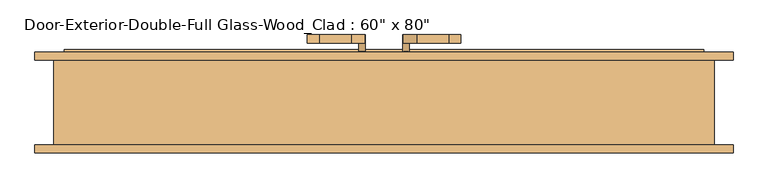
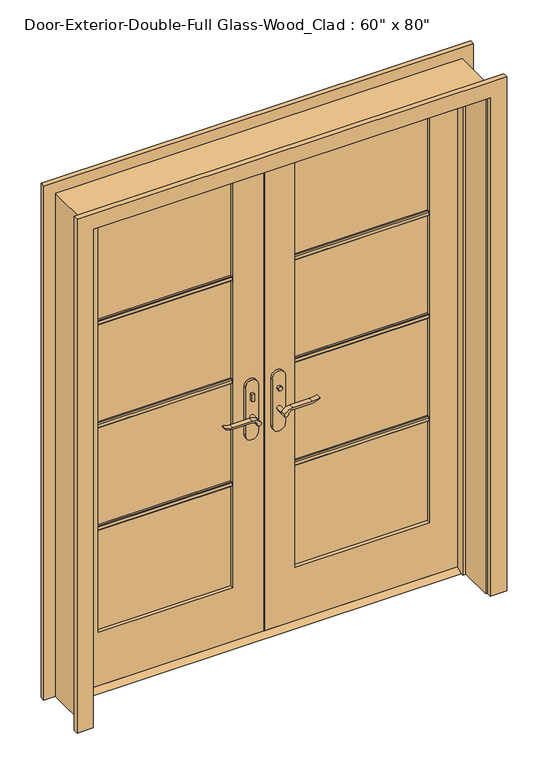
"""IFC4 building model written with IfcOpenShell, lengths in millimetres: door geometry."""

from ifc_helpers import new_model, si_unit, point, frame, frame_2d, origin, place, context, project, spatial, polyline, circle_curve, trimmed, segment, composite_curve, outline, extrude, faceted_brep, source, transform, mapped, element, save


def door_b03bd389(model_context):
    return source(origin(), model_context, "Body", "SolidModel", [
        extrude(outline(polyline([(63.5, 12.7), (98.425, 12.7), (123.825, 0.0), (38.1, 0.0), (63.5, 12.7)])), frame((-762.0, 0.0, 0.0), z_axis=(1.0, 0.0, 0.0), x_axis=(0.0, 1.0, 0.0)), (0.0, 0.0, 1.0), 1524.0),
        extrude(outline(polyline([(-47.4019111, 43.5), (-57.4019111, 43.5), (-57.4019111, 53.5), (-47.4019111, 53.5), (-47.4019111, 43.5)])), frame((0.0, 0.0, 981.9), z_axis=(0.0, 0.0, 1.0), x_axis=(1.0, 0.0, 0.0)), (0.0, 0.0, 1.0), 30.0),
        extrude(outline(composite_curve([segment(trimmed(circle_curve(frame_2d((996.9, -52.4019111)), 8.0), [point((996.9, -60.4019111))], [point((996.9, -44.4019111))], False, "CARTESIAN"), True, "CONTINUOUS"), segment(trimmed(circle_curve(frame_2d((996.9, -52.4019111)), 8.0), [point((996.9, -44.4019111))], [point((996.9, -60.4019111))], False, "CARTESIAN"), True, "CONTINUOUS")], self_intersect=False)), frame((0.0, 108.425, 0.0), z_axis=(0.0, 1.0, 0.0), x_axis=(0.0, 0.0, 1.0)), (0.0, 0.0, 1.0), 10.0),
        extrude(outline(composite_curve([segment(trimmed(circle_curve(frame_2d((897.1555521, -76.0694241)), 37.2832219), [point((919.0523287, -45.8937749))], [point((934.4, -77.7693445))], False, "CARTESIAN"), True, "CONTINUOUS"), segment(polyline([(934.4, -77.7693445), (934.4, -154.045502)]), True, "CONTINUOUS"), segment(trimmed(circle_curve(frame_2d((1017.6850638, -153.9791202)), 83.2850902), [point((934.4, -154.045502))], [point((939.4, -182.4019111))], True, "CARTESIAN"), True, "CONTINUOUS"), segment(polyline([(939.4, -182.4019111), (936.6135558, -182.4019111)]), True, "CONTINUOUS"), segment(trimmed(circle_curve(frame_2d((986.6709207, -150.4622499)), 59.3791355), [point((936.6135558, -182.4019111))], [point((927.4, -154.045502))], False, "CARTESIAN"), True, "CONTINUOUS"), segment(polyline([(927.4, -154.045502), (927.4, -77.7881013)]), True, "CONTINUOUS"), segment(trimmed(circle_curve(frame_2d((909.2738613, -77.7881013)), 18.1261387), [point((927.4, -77.7881013))], [point((914.4, -60.4019111))], True, "CARTESIAN"), True, "CONTINUOUS"), segment(trimmed(circle_curve(frame_2d((914.4, -52.4019111)), 8.0), [point((914.4, -60.4019111))], [point((919.0523287, -45.8937749))], False, "CARTESIAN"), True, "CONTINUOUS")], self_intersect=False)), frame((0.0, 3.5, 0.0), z_axis=(0.0, 1.0, 0.0), x_axis=(0.0, 0.0, 1.0)), (0.0, 0.0, 1.0), 20.0),
        extrude(outline(composite_curve([segment(trimmed(circle_curve(frame_2d((914.4, -52.4019111)), 8.0), [point((914.3999903, -60.4019111))], [point((919.0523287, -45.8937749))], False, "CARTESIAN"), True, "CONTINUOUS"), segment(trimmed(circle_curve(frame_2d((897.1555521, -76.0694241)), 37.2832219), [point((919.0523287, -45.8937749))], [point((934.4, -77.7693445))], False, "CARTESIAN"), True, "CONTINUOUS"), segment(polyline([(934.4, -77.7693445), (934.4, -154.045502)]), True, "CONTINUOUS"), segment(trimmed(circle_curve(frame_2d((1017.6850638, -153.9791202)), 83.2850902), [point((934.4, -154.045502))], [point((939.4, -182.4019111))], True, "CARTESIAN"), True, "CONTINUOUS"), segment(polyline([(939.4, -182.4019111), (936.6135558, -182.4019111)]), True, "CONTINUOUS"), segment(trimmed(circle_curve(frame_2d((986.6709207, -150.4622499)), 59.3791355), [point((936.6135558, -182.4019111))], [point((927.4, -154.045502))], False, "CARTESIAN"), True, "CONTINUOUS"), segment(polyline([(927.4, -154.045502), (927.4, -77.788099)]), True, "CONTINUOUS"), segment(trimmed(circle_curve(frame_2d((909.2738682, -77.788099)), 18.1261318), [point((927.4, -77.788099))], [point((914.3999903, -60.4019111))], True, "CARTESIAN"), True, "CONTINUOUS")], self_intersect=False)), frame((0.0, 138.425, 0.0), z_axis=(0.0, 1.0, 0.0), x_axis=(0.0, 0.0, 1.0)), (0.0, 0.0, 1.0), 20.0),
        extrude(outline(composite_curve([segment(trimmed(circle_curve(frame_2d((914.4, -52.4019111)), 8.0), [point((914.4, -60.4019111))], [point((914.4, -44.4019111))], False, "CARTESIAN"), True, "CONTINUOUS"), segment(trimmed(circle_curve(frame_2d((914.4, -52.4019111)), 8.0), [point((914.4, -44.4019111))], [point((914.4, -60.4019111))], False, "CARTESIAN"), True, "CONTINUOUS")], self_intersect=False)), frame((0.0, 23.5, 0.0), z_axis=(0.0, 1.0, 0.0), x_axis=(0.0, 0.0, 1.0)), (0.0, 0.0, 1.0), 30.0),
        extrude(outline(composite_curve([segment(trimmed(circle_curve(frame_2d((914.4, -52.4019111)), 8.0), [point((914.4, -60.4019111))], [point((914.4, -44.4019111))], False, "CARTESIAN"), True, "CONTINUOUS"), segment(trimmed(circle_curve(frame_2d((914.4, -52.4019111)), 8.0), [point((914.4, -44.4019111))], [point((914.4, -60.4019111))], False, "CARTESIAN"), True, "CONTINUOUS")], self_intersect=False)), frame((0.0, 108.425, 0.0), z_axis=(0.0, 1.0, 0.0), x_axis=(0.0, 0.0, 1.0)), (0.0, 0.0, 1.0), 30.0),
        extrude(outline(composite_curve([segment(polyline([(844.4, -27.4019111), (1039.4, -27.4019111)]), True, "CONTINUOUS"), segment(trimmed(circle_curve(frame_2d((1039.4, -52.4019111)), 25.0), [point((1039.4, -27.4019111))], [point((1039.4, -77.4019111))], False, "CARTESIAN"), True, "CONTINUOUS"), segment(polyline([(1039.4, -77.4019111), (844.4, -77.4019111)]), True, "CONTINUOUS"), segment(trimmed(circle_curve(frame_2d((844.4, -52.4019111)), 25.0), [point((844.4, -77.4019111))], [point((844.4, -27.4019111))], False, "CARTESIAN"), True, "CONTINUOUS")], self_intersect=False)), frame((0.0, 53.5, 0.0), z_axis=(0.0, 1.0, 0.0), x_axis=(0.0, 0.0, 1.0)), (0.0, 0.0, 1.0), 10.0),
        extrude(outline(composite_curve([segment(polyline([(844.4, -27.4019111), (1039.4, -27.4019111)]), True, "CONTINUOUS"), segment(trimmed(circle_curve(frame_2d((1039.4, -52.4019111)), 25.0), [point((1039.4, -27.4019111))], [point((1039.4, -77.4019111))], False, "CARTESIAN"), True, "CONTINUOUS"), segment(polyline([(1039.4, -77.4019111), (844.4, -77.4019111)]), True, "CONTINUOUS"), segment(trimmed(circle_curve(frame_2d((844.4, -52.4019111)), 25.0), [point((844.4, -77.4019111))], [point((844.4, -27.4019111))], False, "CARTESIAN"), True, "CONTINUOUS")], self_intersect=False)), frame((0.0, 98.425, 0.0), z_axis=(0.0, 1.0, 0.0), x_axis=(0.0, 0.0, 1.0)), (0.0, 0.0, 1.0), 10.0),
        extrude(outline(polyline([(47.3875, 118.425), (57.3875, 118.425), (57.3875, 108.425), (47.3875, 108.425), (47.3875, 118.425)])), frame((0.0, 0.0, 981.9), z_axis=(0.0, 0.0, 1.0), x_axis=(1.0, 0.0, 0.0)), (0.0, 0.0, 1.0), 30.0),
        extrude(outline(composite_curve([segment(trimmed(circle_curve(frame_2d((996.9, 52.3875)), 8.0), [point((996.9, 60.3875))], [point((996.9, 44.3875))], False, "CARTESIAN"), True, "CONTINUOUS"), segment(trimmed(circle_curve(frame_2d((996.9, 52.3875)), 8.0), [point((996.9, 44.3875))], [point((996.9, 60.3875))], False, "CARTESIAN"), True, "CONTINUOUS")], self_intersect=False)), frame((0.0, 43.5, 0.0), z_axis=(0.0, 1.0, 0.0), x_axis=(0.0, 0.0, 1.0)), (0.0, 0.0, 1.0), 10.0),
        extrude(outline(composite_curve([segment(trimmed(circle_curve(frame_2d((914.4, 52.3875)), 8.0), [point((919.0523287, 45.8793637))], [point((914.4, 60.3875))], False, "CARTESIAN"), True, "CONTINUOUS"), segment(trimmed(circle_curve(frame_2d((909.2738613, 77.7736901)), 18.1261387), [point((914.4, 60.3875))], [point((927.4, 77.7736901))], True, "CARTESIAN"), True, "CONTINUOUS"), segment(polyline([(927.4, 77.7736901), (927.4, 154.0310909)]), True, "CONTINUOUS"), segment(trimmed(circle_curve(frame_2d((986.6709207, 150.4478388)), 59.3791355), [point((927.4, 154.0310909))], [point((936.6135558, 182.3875))], False, "CARTESIAN"), True, "CONTINUOUS"), segment(polyline([(936.6135558, 182.3875), (939.4, 182.3875)]), True, "CONTINUOUS"), segment(trimmed(circle_curve(frame_2d((1017.6850638, 153.9647091)), 83.2850902), [point((939.4, 182.3875))], [point((934.4, 154.0310909))], True, "CARTESIAN"), True, "CONTINUOUS"), segment(polyline([(934.4, 154.0310909), (934.4, 77.7549333)]), True, "CONTINUOUS"), segment(trimmed(circle_curve(frame_2d((897.1555521, 76.0550129)), 37.2832219), [point((934.4, 77.7549333))], [point((919.0523287, 45.8793637))], False, "CARTESIAN"), True, "CONTINUOUS")], self_intersect=False)), frame((0.0, 138.425, 0.0), z_axis=(0.0, 1.0, 0.0), x_axis=(0.0, 0.0, 1.0)), (0.0, 0.0, 1.0), 20.0),
        extrude(outline(composite_curve([segment(trimmed(circle_curve(frame_2d((909.2738682, 77.7736878)), 18.1261318), [point((914.3999903, 60.3875))], [point((927.4, 77.7736878))], True, "CARTESIAN"), True, "CONTINUOUS"), segment(polyline([(927.4, 77.7736878), (927.4, 154.0310909)]), True, "CONTINUOUS"), segment(trimmed(circle_curve(frame_2d((986.6709207, 150.4478388)), 59.3791355), [point((927.4, 154.0310909))], [point((936.6135558, 182.3875))], False, "CARTESIAN"), True, "CONTINUOUS"), segment(polyline([(936.6135558, 182.3875), (939.4, 182.3875)]), True, "CONTINUOUS"), segment(trimmed(circle_curve(frame_2d((1017.6850638, 153.9647091)), 83.2850902), [point((939.4, 182.3875))], [point((934.4, 154.0310909))], True, "CARTESIAN"), True, "CONTINUOUS"), segment(polyline([(934.4, 154.0310909), (934.4, 77.7549333)]), True, "CONTINUOUS"), segment(trimmed(circle_curve(frame_2d((897.1555521, 76.0550129)), 37.2832219), [point((934.4, 77.7549333))], [point((919.0523287, 45.8793637))], False, "CARTESIAN"), True, "CONTINUOUS"), segment(trimmed(circle_curve(frame_2d((914.4, 52.3875)), 8.0), [point((919.0523287, 45.8793637))], [point((914.3999903, 60.3875))], False, "CARTESIAN"), True, "CONTINUOUS")], self_intersect=False)), frame((0.0, 3.5, 0.0), z_axis=(0.0, 1.0, 0.0), x_axis=(0.0, 0.0, 1.0)), (0.0, 0.0, 1.0), 20.0),
        extrude(outline(composite_curve([segment(trimmed(circle_curve(frame_2d((914.4, 52.3875)), 8.0), [point((914.4, 60.3875))], [point((914.4, 44.3875))], False, "CARTESIAN"), True, "CONTINUOUS"), segment(trimmed(circle_curve(frame_2d((914.4, 52.3875)), 8.0), [point((914.4, 44.3875))], [point((914.4, 60.3875))], False, "CARTESIAN"), True, "CONTINUOUS")], self_intersect=False)), frame((0.0, 108.425, 0.0), z_axis=(0.0, 1.0, 0.0), x_axis=(0.0, 0.0, 1.0)), (0.0, 0.0, 1.0), 30.0),
        extrude(outline(composite_curve([segment(trimmed(circle_curve(frame_2d((914.4, 52.3875)), 8.0), [point((914.4, 60.3875))], [point((914.4, 44.3875))], False, "CARTESIAN"), True, "CONTINUOUS"), segment(trimmed(circle_curve(frame_2d((914.4, 52.3875)), 8.0), [point((914.4, 44.3875))], [point((914.4, 60.3875))], False, "CARTESIAN"), True, "CONTINUOUS")], self_intersect=False)), frame((0.0, 23.5, 0.0), z_axis=(0.0, 1.0, 0.0), x_axis=(0.0, 0.0, 1.0)), (0.0, 0.0, 1.0), 30.0),
        extrude(outline(composite_curve([segment(trimmed(circle_curve(frame_2d((844.4, 52.3875)), 25.0), [point((844.4, 27.3875))], [point((844.4, 77.3875))], False, "CARTESIAN"), True, "CONTINUOUS"), segment(polyline([(844.4, 77.3875), (1039.4, 77.3875)]), True, "CONTINUOUS"), segment(trimmed(circle_curve(frame_2d((1039.4, 52.3875)), 25.0), [point((1039.4, 77.3875))], [point((1039.4, 27.3875))], False, "CARTESIAN"), True, "CONTINUOUS"), segment(polyline([(1039.4, 27.3875), (844.4, 27.3875)]), True, "CONTINUOUS")], self_intersect=False)), frame((0.0, 98.425, 0.0), z_axis=(0.0, 1.0, 0.0), x_axis=(0.0, 0.0, 1.0)), (0.0, 0.0, 1.0), 10.0),
        extrude(outline(composite_curve([segment(trimmed(circle_curve(frame_2d((844.4, 52.3875)), 25.0), [point((844.4, 27.3875))], [point((844.4, 77.3875))], False, "CARTESIAN"), True, "CONTINUOUS"), segment(polyline([(844.4, 77.3875), (1039.4, 77.3875)]), True, "CONTINUOUS"), segment(trimmed(circle_curve(frame_2d((1039.4, 52.3875)), 25.0), [point((1039.4, 77.3875))], [point((1039.4, 27.3875))], False, "CARTESIAN"), True, "CONTINUOUS"), segment(polyline([(1039.4, 27.3875), (844.4, 27.3875)]), True, "CONTINUOUS")], self_intersect=False)), frame((0.0, 53.5, 0.0), z_axis=(0.0, 1.0, 0.0), x_axis=(0.0, 0.0, 1.0)), (0.0, 0.0, 1.0), 10.0),
        extrude(outline(polyline([(77.47, 1502.171875), (77.47, 1483.121875), (71.12, 1483.121875), (67.945, 1486.296875), (67.945, 1498.996875), (71.12, 1502.171875), (77.47, 1502.171875)])), frame((120.65, 0.0, 0.0), z_axis=(1.0, 0.0, 0.0), x_axis=(0.0, 1.0, 0.0)), (0.0, 0.0, 1.0), 520.7),
        extrude(outline(polyline([(77.47, 1081.88125), (77.47, 1062.83125), (71.12, 1062.83125), (67.945, 1066.00625), (67.945, 1078.70625), (71.12, 1081.88125), (77.47, 1081.88125)])), frame((120.65, 0.0, 0.0), z_axis=(1.0, 0.0, 0.0), x_axis=(0.0, 1.0, 0.0)), (0.0, 0.0, 1.0), 520.7),
        extrude(outline(polyline([(77.47, 661.590625), (77.47, 642.540625), (71.12, 642.540625), (67.945, 645.715625), (67.945, 658.415625), (71.12, 661.590625), (77.47, 661.590625)])), frame((120.65, 0.0, 0.0), z_axis=(1.0, 0.0, 0.0), x_axis=(0.0, 1.0, 0.0)), (0.0, 0.0, 1.0), 520.7),
        extrude(outline(polyline([(84.455, 1502.171875), (90.805, 1502.171875), (93.98, 1498.996875), (93.98, 1486.296875), (90.805, 1483.121875), (84.455, 1483.121875), (84.455, 1502.171875)])), frame((-641.35, 0.0, 0.0), z_axis=(1.0, 0.0, 0.0), x_axis=(0.0, 1.0, 0.0)), (0.0, 0.0, 1.0), 520.7),
        extrude(outline(polyline([(84.455, 1081.88125), (90.805, 1081.88125), (93.98, 1078.70625), (93.98, 1066.00625), (90.805, 1062.83125), (84.455, 1062.83125), (84.455, 1081.88125)])), frame((-641.35, 0.0, 0.0), z_axis=(1.0, 0.0, 0.0), x_axis=(0.0, 1.0, 0.0)), (0.0, 0.0, 1.0), 520.7),
        extrude(outline(polyline([(84.455, 661.590625), (90.805, 661.590625), (93.98, 658.415625), (93.98, 645.715625), (90.805, 642.540625), (84.455, 642.540625), (84.455, 661.590625)])), frame((-641.35, 0.0, 0.0), z_axis=(1.0, 0.0, 0.0), x_axis=(0.0, 1.0, 0.0)), (0.0, 0.0, 1.0), 520.7),
        extrude(outline(polyline([(84.455, 1502.171875), (90.805, 1502.171875), (93.98, 1498.996875), (93.98, 1486.296875), (90.805, 1483.121875), (84.455, 1483.121875), (84.455, 1502.171875)])), frame((120.65, 0.0, 0.0), z_axis=(1.0, 0.0, 0.0), x_axis=(0.0, 1.0, 0.0)), (0.0, 0.0, 1.0), 520.7),
        extrude(outline(polyline([(84.455, 1081.88125), (90.805, 1081.88125), (93.98, 1078.70625), (93.98, 1066.00625), (90.805, 1062.83125), (84.455, 1062.83125), (84.455, 1081.88125)])), frame((120.65, 0.0, 0.0), z_axis=(1.0, 0.0, 0.0), x_axis=(0.0, 1.0, 0.0)), (0.0, 0.0, 1.0), 520.7),
        extrude(outline(polyline([(84.455, 661.590625), (90.805, 661.590625), (93.98, 658.415625), (93.98, 645.715625), (90.805, 642.540625), (84.455, 642.540625), (84.455, 661.590625)])), frame((120.65, 0.0, 0.0), z_axis=(1.0, 0.0, 0.0), x_axis=(0.0, 1.0, 0.0)), (0.0, 0.0, 1.0), 520.7),
        extrude(outline(polyline([(77.47, 1502.171875), (77.47, 1483.121875), (71.12, 1483.121875), (67.945, 1486.296875), (67.945, 1498.996875), (71.12, 1502.171875), (77.47, 1502.171875)])), frame((-641.35, 0.0, 0.0), z_axis=(1.0, 0.0, 0.0), x_axis=(0.0, 1.0, 0.0)), (0.0, 0.0, 1.0), 520.7),
        extrude(outline(polyline([(77.47, 1081.88125), (77.47, 1062.83125), (71.12, 1062.83125), (67.945, 1066.00625), (67.945, 1078.70625), (71.12, 1081.88125), (77.47, 1081.88125)])), frame((-641.35, 0.0, 0.0), z_axis=(1.0, 0.0, 0.0), x_axis=(0.0, 1.0, 0.0)), (0.0, 0.0, 1.0), 520.7),
        extrude(outline(polyline([(77.47, 661.590625), (77.47, 642.540625), (71.12, 642.540625), (67.945, 645.715625), (67.945, 658.415625), (71.12, 661.590625), (77.47, 661.590625)])), frame((-641.35, 0.0, 0.0), z_axis=(1.0, 0.0, 0.0), x_axis=(0.0, 1.0, 0.0)), (0.0, 0.0, 1.0), 520.7),
        extrude(outline(polyline([(0.0, 768.35), (0.0, 831.85), (2101.85, 831.85), (2101.85, -831.85), (0.0, -831.85), (0.0, -768.35), (2038.35, -768.35), (2038.35, 768.35), (0.0, 768.35)])), frame((0.0, 98.425, 0.0), z_axis=(0.0, 1.0, 0.0), x_axis=(0.0, 0.0, 1.0)), (0.0, 0.0, 1.0), 19.05),
        extrude(outline(polyline([(0.0, 768.35), (0.0, 831.85), (2101.85, 831.85), (2101.85, -831.85), (0.0, -831.85), (0.0, -768.35), (2038.35, -768.35), (2038.35, 768.35), (0.0, 768.35)])), frame((0.0, -123.825, 0.0), z_axis=(0.0, 1.0, 0.0), x_axis=(0.0, 0.0, 1.0)), (0.0, 0.0, 1.0), 19.05),
        extrude(outline(polyline([(12.7, 762.0), (2032.0, 762.0), (2032.0, 1.5875), (12.7, 1.5875), (12.7, 762.0)]), holes=[polyline([(1912.9375, 120.65), (1912.9375, 641.35), (231.775, 641.35), (231.775, 120.65), (1912.9375, 120.65)])]), frame((0.0, 63.5, 0.0), z_axis=(0.0, 1.0, 0.0), x_axis=(0.0, 0.0, 1.0)), (0.0, 0.0, 1.0), 34.925),
        extrude(outline(polyline([(2032.0, -762.0), (12.7, -762.0), (12.7, -1.6019111), (2032.0, -1.6019111), (2032.0, -762.0)]), holes=[polyline([(231.775, -641.35), (1912.9375, -641.35), (1912.9375, -120.65), (231.775, -120.65), (231.775, -641.35)])]), frame((0.0, 63.5, 0.0), z_axis=(0.0, 1.0, 0.0), x_axis=(0.0, 0.0, 1.0)), (0.0, 0.0, 1.0), 34.925),
        faceted_brep([(787.4, 98.425, 0.0), (787.4, -104.775, 0.0), (762.0, -104.775, 0.0), (762.0, 28.575, 0.0), (749.3, 28.575, 0.0), (749.3, 63.5, 0.0), (762.0, 63.5, 0.0), (762.0, 98.425, 0.0), (787.4, 98.425, 2057.4), (787.4, -104.775, 2057.4), (-787.4, -104.775, 2057.4), (-787.4, -104.775, 0.0), (-762.0, -104.775, 0.0), (-762.0, -104.775, 2032.0), (762.0, -104.775, 2032.0), (762.0, 28.575, 2032.0), (-762.0, 28.575, 2032.0), (-762.0, 28.575, 0.0), (-749.3, 28.575, 0.0), (-749.3, 28.575, 2019.3), (749.3, 28.575, 2019.3), (749.3, 63.5, 2019.3), (1.5875, 63.5, 2019.3), (-1.6019111, 63.5, 2019.3), (-749.3, 63.5, 2019.3), (-749.3, 63.5, 0.0), (-762.0, 63.5, 0.0), (-762.0, 63.5, 2032.0), (-1.6019111, 63.5, 2032.0), (1.5875, 63.5, 2032.0), (762.0, 63.5, 2032.0), (762.0, 98.425, 2032.0), (1.5875, 98.425, 2032.0), (-1.6019111, 98.425, 2032.0), (-762.0, 98.425, 2032.0), (-762.0, 98.425, 0.0), (-787.4, 98.425, 0.0), (-787.4, 98.425, 2057.4)], [[[0, 1, 2, 3, 4, 5, 6, 7]], [[1, 0, 8, 9]], [[2, 1, 9, 10, 11, 12, 13, 14]], [[3, 2, 14, 15]], [[4, 3, 15, 16, 17, 18, 19, 20]], [[5, 4, 20, 21]], [[6, 5, 21, 22, 23, 24, 25, 26, 27, 28, 29, 30]], [[7, 6, 30, 31]], [[0, 7, 31, 32, 33, 34, 35, 36, 37, 8]], [[9, 8, 37, 10]], [[14, 13, 16, 15]], [[20, 19, 24, 23, 22, 21]], [[31, 30, 29, 28, 27, 34, 33, 32]], [[12, 11, 36, 35, 26, 25, 18, 17]], [[11, 10, 37, 36]], [[13, 12, 17, 16]], [[19, 18, 25, 24]], [[27, 26, 35, 34]]]),
        extrude(outline(polyline([(641.35, 77.47), (120.65, 77.47), (120.65, 84.455), (641.35, 84.455), (641.35, 77.47)])), frame((0.0, 0.0, 231.775), z_axis=(0.0, 0.0, 1.0), x_axis=(1.0, 0.0, 0.0)), (0.0, 0.0, 1.0), 1681.1625),
        extrude(outline(polyline([(-120.65, 77.47), (-641.35, 77.47), (-641.35, 84.455), (-120.65, 84.455), (-120.65, 77.47)])), frame((0.0, 0.0, 231.775), z_axis=(0.0, 0.0, 1.0), x_axis=(1.0, 0.0, 0.0)), (0.0, 0.0, 1.0), 1681.1625),
    ])


if __name__ == "__main__":
    model = new_model("IFC4")
    model_context = context("Model", 3, world=origin())
    ifc_project = project(units=[si_unit("LENGTHUNIT", "METRE", prefix="MILLI")], contexts=[model_context])
    site = spatial("IfcSite", under=ifc_project)
    building = spatial("IfcBuilding", under=site)
    placement = place(None, origin())
    door_shape = door_b03bd389(model_context)
    element("IfcDoor", 1, ObjectType="Door-Exterior-Double-Full Glass-Wood_Clad : 60\" x 80\"", at=placement, inside=building, context=model_context, shape_type="MappedRepresentation", body=[
        mapped(door_shape, transform((0.0, 0.0, 0.0), x_axis=(1.0, 0.0, 0.0), y_axis=(0.0, 1.0, 0.0), z_axis=(0.0, 0.0, 1.0))),
    ])
    save(model, "model.ifc")

# Revit data of these elements
# Type "Door-Exterior-Double-Full Glass-Wood_Clad : 60\" x 80\""
#   Type Mark = "9"
#   Assembly Code = "B2030100"
#   Analytic Construction = "French door, wood frame with double glass"
#   Top Rail = 0' - 4 11/16"
#   Threshold Offset [instance default] = 0' - 0 1/2"
#   Thickness = 0' - 1 3/8"
#   Thermal Resistance (R) = 1.9158 (h·ft²·°F)/BTU
#   Swing Angle [instance default] = 90.00°
#   Stiles = 0' - 4 3/4"
#   Rough Width = 5' - 2"
#   Rough Height = 6' - 9"
#   Panel Width = 2' - 6"
#   Door Offset [instance default] = 0' - 0"
#   Height = 6' - 8"
#   Width = 5' - 0"
#   Heat Transfer Coefficient (U) = 0.5220 BTU/(h·ft²·°F)
#   Bottom Rail = 0' - 9 1/8"
#   Exterior Trim [instance default] = yes
#   Threshold [instance default] = yes
#   Show Grill [instance default] = yes
#   Function = 1
#   Trim Material = Cherry
#   Threshold Material = Cherry
#   Panel Material = Cherry
#   Glazing = Glass
#   Frame Material = Cherry
#   Door Handle Material = Aluminum
#   Visual Light Transmittance = 0
#   Solar Heat Gain Coefficient = 0
#   Wall Closure = (empty or 0)
#   Construction Type = (empty or 0)
# Element 1 (IfcDoor, "Door-Exterior-Double-Full Glass-Wood_Clad : 60\" x 80\"")
#   Materials on its faces: "Cherry", "Aluminum", "Glass"
# Materials
#   "Cherry": class "Wood", colour RGB 226 177 128, transparency 0, Description = "Prunus Serotina", Cost = 0
#   "Glass": class "Glass", colour RGB 0 128 192, transparency 0.75, Description = "Soda Lime Glass", Cost = 0
#   "Aluminum": class "Metal", colour RGB 247 247 247, transparency 0, Description = "Aluminum 6061", Cost = 0
